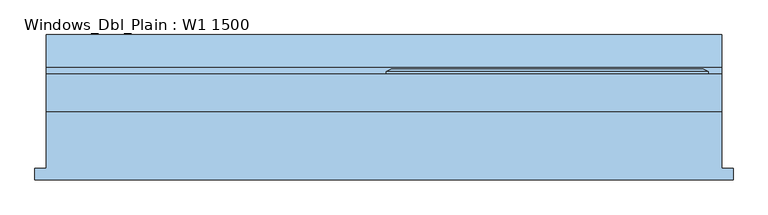
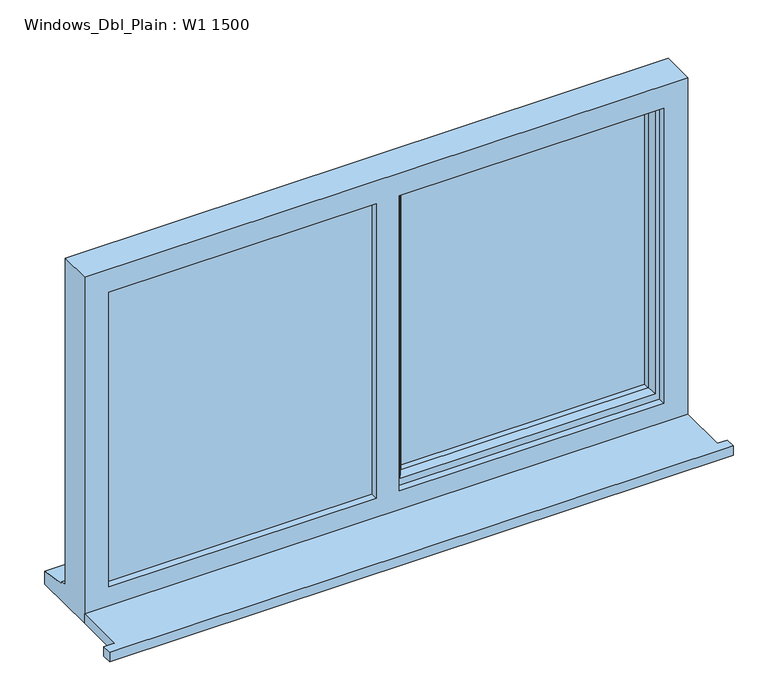
"""IFC4 building model written with IfcOpenShell, lengths in millimetres: window geometry, Windows_Dbl_Plain : W1 1500."""

from ifc_helpers import new_model, si_unit, frame, origin, place, context, project, spatial, polyline, outline, extrude, faceted_brep, source, transform, mapped, element, save


def windows_dbl_plain_w1_1500_219ff321(model_context):
    return source(origin(), model_context, "Body", "SolidModel", [
        extrude(outline(polyline([(-1060.0, -146.5434322), (-1060.0, -121.5434322), (-1035.0, -121.5434322), (-1035.0, 5.4565678), (465.0, 5.4565678), (465.0, -121.5434322), (490.0, -121.5434322), (490.0, -146.5434322), (-1060.0, -146.5434322)])), frame((0.0, 0.0, 1200.0), z_axis=(0.0, 0.0, 1.0), x_axis=(1.0, 0.0, 0.0)), (0.0, 0.0, 1.0), 25.0),
        faceted_brep([(-280.0, 88.4565678, 2080.0), (-280.0, 94.2300705, 2080.0), (-280.0, 94.2300705, 1253.0), (-280.0, 88.4565678, 1253.0), (-270.0, 23.4565678, 2070.0), (-270.0, 88.4565678, 2070.0), (-270.0, 88.4565678, 1263.0), (-270.0, 23.4565678, 1263.0), (-230.0, 37.9494677, 2030.0), (-240.1480377, 23.4565678, 2040.1480377), (-240.1480377, 23.4565678, 1292.8519623), (-230.0, 37.9494677, 1303.0), (-230.0, 52.4565678, 2030.0), (-230.0, 52.4565678, 1303.0), (-240.0, 76.4565678, 2040.0), (-240.0, 52.4565678, 2040.0), (-240.0, 52.4565678, 1293.0), (-240.0, 76.4565678, 1293.0), (-230.0, 94.2300705, 2030.0), (-230.0, 76.4565678, 2030.0), (-230.0, 76.4565678, 1303.0), (-230.0, 94.2300705, 1303.0), (-247.4457548, 100.0035732, 2047.4457548), (-247.4457548, 100.0035732, 1285.5542452), (-269.2153903, 100.0035732, 2069.2153903), (-269.2153903, 100.0035732, 1263.7846097), (435.0, 94.2300705, 1253.0), (435.0, 88.4565678, 1253.0), (425.0, 88.4565678, 1263.0), (425.0, 23.4565678, 1263.0), (395.1480377, 23.4565678, 1292.8519623), (385.0, 37.9494677, 1303.0), (385.0, 52.4565678, 1303.0), (395.0, 52.4565678, 1293.0), (395.0, 76.4565678, 1293.0), (385.0, 76.4565678, 1303.0), (385.0, 94.2300705, 1303.0), (402.4457548, 100.0035732, 1285.5542452), (424.2153903, 100.0035732, 1263.7846097), (435.0, 94.2300705, 2080.0), (435.0, 88.4565678, 2080.0), (425.0, 88.4565678, 2070.0), (425.0, 23.4565678, 2070.0), (395.1480377, 23.4565678, 2040.1480377), (385.0, 37.9494677, 2030.0), (385.0, 52.4565678, 2030.0), (395.0, 52.4565678, 2040.0), (395.0, 76.4565678, 2040.0), (385.0, 76.4565678, 2030.0), (385.0, 94.2300705, 2030.0), (402.4457548, 100.0035732, 2047.4457548), (424.2153903, 100.0035732, 2069.2153903)], [[[0, 1, 2, 3]], [[4, 5, 6, 7]], [[8, 9, 10, 11]], [[12, 8, 11, 13]], [[14, 15, 16, 17]], [[18, 19, 20, 21]], [[22, 18, 21, 23]], [[1, 24, 25, 2]], [[3, 2, 26, 27]], [[7, 6, 28, 29]], [[11, 10, 30, 31]], [[13, 11, 31, 32]], [[17, 16, 33, 34]], [[21, 20, 35, 36]], [[23, 21, 36, 37]], [[2, 25, 38, 26]], [[27, 26, 39, 40]], [[29, 28, 41, 42]], [[31, 30, 43, 44]], [[32, 31, 44, 45]], [[34, 33, 46, 47]], [[36, 35, 48, 49]], [[37, 36, 49, 50]], [[26, 38, 51, 39]], [[40, 39, 1, 0]], [[3, 27, 40, 0], [5, 41, 28, 6]], [[42, 41, 5, 4]], [[7, 29, 42, 4], [9, 43, 30, 10]], [[44, 43, 9, 8]], [[45, 44, 8, 12]], [[15, 46, 33, 16], [13, 32, 45, 12]], [[47, 46, 15, 14]], [[17, 34, 47, 14], [19, 48, 35, 20]], [[49, 48, 19, 18]], [[50, 49, 18, 22]], [[24, 51, 38, 25], [23, 37, 50, 22]], [[39, 51, 24, 1]]]),
        extrude(outline(polyline([(2050.0, -310.0), (2070.0, -310.0), (2070.0, -995.0), (1263.0, -995.0), (1263.0, -310.0), (1283.0, -310.0), (1283.0, -975.0), (2050.0, -975.0), (2050.0, -310.0)])), frame((0.0, 47.4565678, 0.0), z_axis=(0.0, 1.0, 0.0), x_axis=(0.0, 0.0, 1.0)), (0.0, 0.0, 1.0), 41.0),
        faceted_brep([(465.0, 5.4565678, 2110.0), (-1035.0, 5.4565678, 2110.0), (-1035.0, 5.4565678, 1200.0), (465.0, 5.4565678, 1200.0), (405.0, 5.4565678, 2050.0), (405.0, 5.4565678, 1275.0), (-252.0, 5.4565678, 1275.0), (-252.0, 5.4565678, 2050.0), (-310.0, 5.4565678, 2050.0), (-310.0, 5.4565678, 1275.0), (-975.0, 5.4565678, 1275.0), (-975.0, 5.4565678, 2050.0), (-1035.0, 88.4565678, 2110.0), (-1035.0, 88.4565678, 1251.0), (-1035.0, 103.4565678, 1249.68767), (-1035.0, 103.4565678, 1244.7449676), (-1035.0, 175.9565678, 1233.8088847), (-1035.0, 175.9565678, 1200.0), (465.0, 88.4565678, 2110.0), (465.0, 88.4565678, 1251.0), (-995.0, 88.4565678, 2070.0), (-995.0, 88.4565678, 1263.0), (-310.0, 88.4565678, 1263.0), (-310.0, 88.4565678, 2070.0), (-270.0, 88.4565678, 2070.0), (-270.0, 88.4565678, 1263.0), (425.0, 88.4565678, 1263.0), (425.0, 88.4565678, 2070.0), (-995.0, 23.4565678, 2070.0), (-995.0, 23.4565678, 1263.0), (-300.0, 23.4565678, 2070.0), (-300.0, 23.4565678, 1263.0), (-310.0, 23.4565678, 2050.0), (-975.0, 23.4565678, 2050.0), (-975.0, 23.4565678, 1275.0), (-310.0, 23.4565678, 1275.0), (-270.0, 23.4565678, 2070.0), (425.0, 23.4565678, 2070.0), (425.0, 23.4565678, 1263.0), (-270.0, 23.4565678, 1263.0), (405.0, 23.4565678, 2050.0), (-252.0, 23.4565678, 2050.0), (-252.0, 23.4565678, 1275.0), (405.0, 23.4565678, 1275.0), (-310.0, 47.4565678, 2070.0), (-300.0, 47.4565678, 2070.0), (465.0, 175.9565678, 1200.0), (465.0, 175.9565678, 1233.8088847), (465.0, 103.4565678, 1244.7449676), (465.0, 103.4565678, 1249.68767), (-300.0, 47.4565678, 1263.0), (-310.0, 47.4565678, 1263.0)], [[[0, 1, 2, 3], [4, 5, 6, 7], [8, 9, 10, 11]], [[2, 1, 12, 13, 14, 15, 16, 17]], [[13, 12, 18, 19], [20, 21, 22, 23], [24, 25, 26, 27]], [[21, 20, 28, 29]], [[28, 30, 31, 29], [32, 33, 34, 35]], [[36, 37, 38, 39], [40, 41, 42, 43]], [[33, 11, 10, 34]], [[1, 0, 18, 12]], [[28, 20, 23, 44, 45, 30]], [[27, 37, 36, 24]], [[11, 33, 32, 8]], [[40, 4, 7, 41]], [[19, 18, 0, 3, 46, 47, 48, 49]], [[27, 26, 38, 37]], [[4, 40, 43, 5]], [[45, 50, 31, 30]], [[50, 45, 44, 51]], [[51, 44, 23, 22]], [[25, 24, 36, 39]], [[41, 7, 6, 42]], [[8, 32, 35, 9]], [[46, 3, 2, 17]], [[47, 46, 17, 16]], [[48, 47, 16, 15]], [[49, 48, 15, 14]], [[19, 49, 14, 13]], [[22, 21, 29, 31, 50, 51]], [[26, 25, 39, 38]], [[6, 5, 43, 42]], [[35, 34, 10, 9]]]),
        extrude(outline(polyline([(-995.0, 47.4565678), (-300.0, 47.4565678), (-300.0, 23.4565678), (-995.0, 23.4565678), (-995.0, 47.4565678)])), frame((0.0, 0.0, 1263.0), z_axis=(0.0, 0.0, 1.0), x_axis=(1.0, 0.0, 0.0)), (0.0, 0.0, 1.0), 807.0),
        extrude(outline(polyline([(395.0, 52.4565678), (-240.0, 52.4565678), (-240.0, 76.4565678), (395.0, 76.4565678), (395.0, 52.4565678)])), frame((0.0, 0.0, 1293.0), z_axis=(0.0, 0.0, 1.0), x_axis=(1.0, 0.0, 0.0)), (0.0, 0.0, 1.0), 747.0),
    ])


if __name__ == "__main__":
    model = new_model("IFC4")
    model_context = context("Model", 3, world=origin())
    ifc_project = project(units=[si_unit("LENGTHUNIT", "METRE", prefix="MILLI")], contexts=[model_context])
    site = spatial("IfcSite", under=ifc_project)
    building = spatial("IfcBuilding", under=site)
    placement = place(None, origin())
    windows_dbl_plain_w1_1500_shape = windows_dbl_plain_w1_1500_219ff321(model_context)
    element("IfcWindow", 1, ObjectType="Windows_Dbl_Plain : W1 1500", at=placement, inside=building, context=model_context, shape_type="MappedRepresentation", body=[
        mapped(windows_dbl_plain_w1_1500_shape, transform((0.0, 0.0, 0.0), x_axis=(1.0, 0.0, 0.0), y_axis=(0.0, 1.0, 0.0), z_axis=(0.0, 0.0, 1.0))),
    ])
    save(model, "model.ifc")

# Revit data of these elements
# Type "Windows_Dbl_Plain : W1 1500"
#   Type Mark = "62"
#   Operation = "DoublePanelVertical"
#   Construction Type Id = "GSP4R"
#   Manufacturer = "Revit"
#   Keynote = "L10"
#   Analytic Construction = "1/8 in Pilkington single glazing"
#   Wrap Layers (Ext) from Ext = 102.5 mm
#   Wrap Layers (Int) from Ext = 177.5 mm
#   Window Board Projection = 25 mm
#   Window Board Extension = 25 mm
#   Visual Light Transmittance = 0.9
#   Solar Heat Gain Coefficient = 0.78
#   Rough Width = 1500 mm
#   Rough Height = 910 mm
#   Height = 910 mm
#   Width = 1500 mm
#   Heat Transfer Coefficient (U) = 3.6886 W/(m²·K)
#   Glazing Thickness = 24 mm
#   FrameOffset - External = 50 mm
#   Frame Depth = 65 mm
#   Default Head Height = 2110 mm
#   Cill Depth = 87.5 mm
#   Cavity Closer Width = 50 mm
#   Cavity Closer Offset from Ext = 102.5 mm
#   Cavity Closer Depth = 85 mm
#   Vis - Cavity Closers = yes
#   Define Thermal Properties by = 1
#   Material Trim = Window Frame
#   Material Glass = Glass
#   Material Frame = Window Frame
#   Wall Closure = (empty or 0)
# Element 1 (IfcWindow, "Windows_Dbl_Plain : W1 1500")
#   Materials on its faces: "Window Frame", "Glass"
# Materials
#   "Window Frame": colour RGB 249 249 249, transparency 0, Keynote = "L10", Cost = 0
#   "Glass": class "Glass", colour RGB 0 128 192, transparency 0.9, Description = "Soda Lime Glass", Cost = 0
